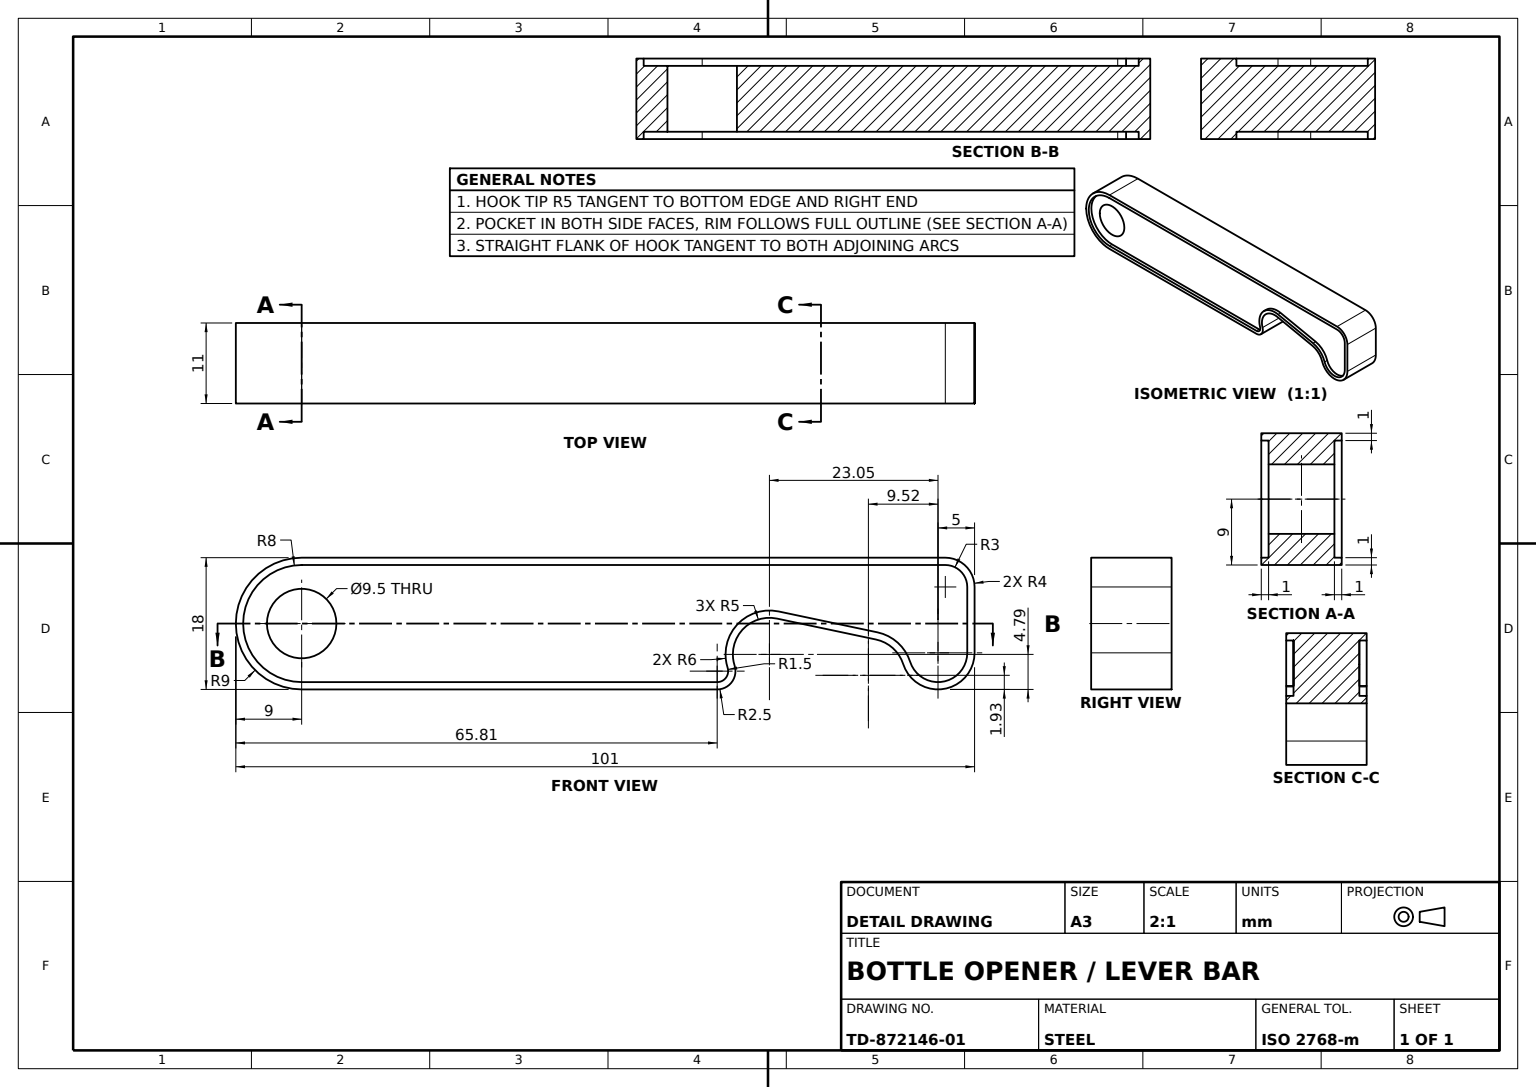
from build123d import *

# Parameters (mm, degrees)
HOOK_BODY_9MM_DEPTH  = 4.5
FACE_START           = 1
FACE_RIM_1MM_DEPTH   = 1
PIVOT_HOLE_SKETCH_R  = 4.75
PIVOT_HOLE_9_5_DEPTH = 16


with BuildPart() as part:
    # Hook Profile Sketch → Hook Body 9mm (new, symmetric)
    with BuildSketch(Plane.XY):
        with BuildLine():
            ThreePointArc((59.190310748, -5.737574987), (60.241407469, -0.861514942), (64.985519507, 0.679318228))
            Line((64.985519507, 0.679318228), (78.516642548, -2.179006643))
            ThreePointArc((78.516642548, -2.179006643), (80.8302907, -3.356581429), (82.241621785, -5.535524915))
            ThreePointArc((82.241621785, -5.535524915), (84.057010413, -8.042129672), (87, -9))
            ThreePointArc((87, -9), (90.535533906, -7.535533906), (92, -4))
            Line((92, -4), (92, 5))
            ThreePointArc((92, 5), (90.828427125, 7.828427125), (88, 9))
            Line((88, 9), (0, 9))
            ThreePointArc((0, 9), (-9, 0), (0, -9))
            Line((0, -9), (56.809405857, -9))
            ThreePointArc((56.809405857, -9), (58.828819452, -7.973760066), (59.190310748, -5.737574987))
        make_face()
    extrude(amount=HOOK_BODY_9MM_DEPTH, both=True)

    # Face Rim Sketch → Face Rim 1mm (add)
    with BuildSketch(Plane.XY.offset(4.5).offset(FACE_START)):
        with BuildLine():
            Line((64.985519507, 0.679318228), (78.516642548, -2.179006643))
            ThreePointArc((78.516642548, -2.179006643), (80.8302907, -3.356581429), (82.241621785, -5.535524915))
            ThreePointArc((82.241621785, -5.535524915), (87.777209408, -8.939225196), (92, -4))
            Line((92, -4), (92, 5))
            ThreePointArc((92, 5), (90.828427125, 7.828427125), (88, 9))
            Line((88, 9), (0, 9))
            ThreePointArc((0, 9), (-9, 0), (0, -9))
            Line((0, -9), (56.809405857, -9))
            ThreePointArc((56.809405857, -9), (58.828819452, -7.973760066), (59.190310748, -5.737574987))
            ThreePointArc((59.190310748, -5.737574987), (60.241407469, -0.861514942), (64.985519507, 0.679318228))
        make_face()
        with BuildLine():
            Line((65.192199302, 1.657726865), (78.723322343, -1.200598005))
            ThreePointArc((78.723322343, -1.200598005), (81.499700126, -2.613687748), (83.193297428, -5.228419932))
            ThreePointArc((83.193297428, -5.228419932), (87.621767526, -7.951380157), (91, -4))
            Line((91, -4), (91, 5))
            ThreePointArc((91, 5), (90.121320344, 7.121320344), (88, 8))
            Line((88, 8), (0, 8))
            ThreePointArc((0, 8), (-8, 0), (0, -8))
            Line((0, -8), (56.809405857, -8))
            ThreePointArc((56.809405857, -8), (58.021054014, -7.38425604), (58.237948791, -6.042544992))
            ThreePointArc((58.237948791, -6.042544992), (59.499264857, -0.191272938), (65.192199302, 1.657726865))
        make_face(mode=Mode.SUBTRACT)
    face_rim_1mm = extrude(amount=-FACE_RIM_1MM_DEPTH)

    # Face Rim Mirror: Face Rim 1mm across plane
    add(face_rim_1mm.mirror(Plane.XY))

    # Pivot Hole Sketch → Pivot Hole Ø9.5 (cut)
    with BuildSketch(Plane(origin=(0, 0, -4.5), x_dir=(-1, 0, 0), z_dir=(0, 0, -1))):
        Circle(PIVOT_HOLE_SKETCH_R)
    extrude(amount=-PIVOT_HOLE_9_5_DEPTH, mode=Mode.SUBTRACT)


solid = part.part
